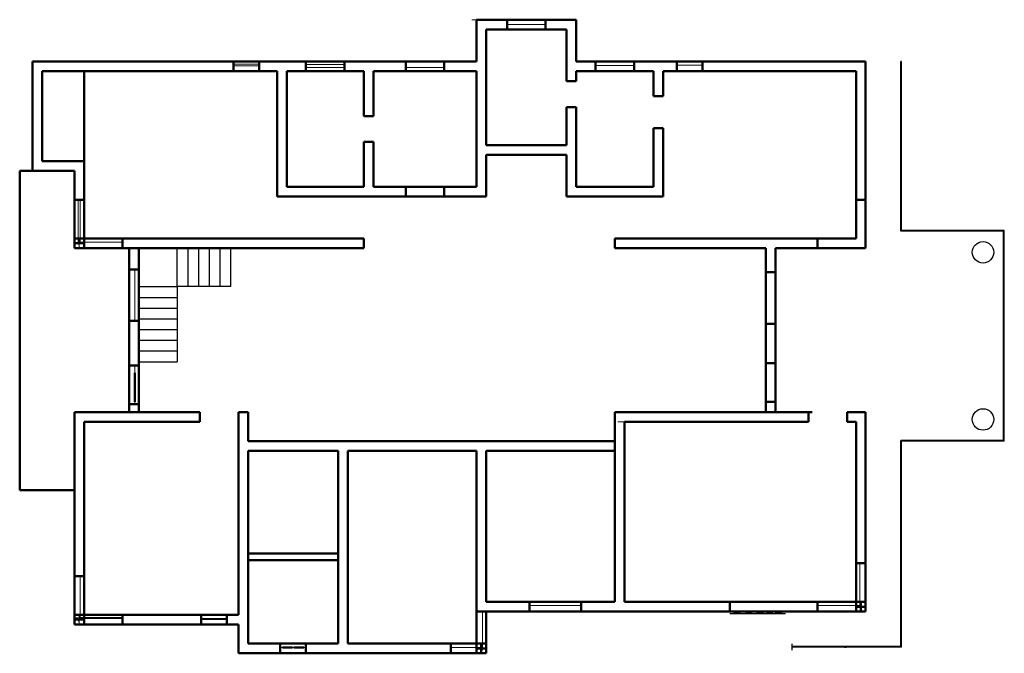
# Model space of a CAD drawing. Units: inches. Extents: x -3 to 916, y -523 to 68.
import ezdxf

# ---------------------------------------------------------------- set-up
doc = ezdxf.new("R2010")
doc.units = ezdxf.units.IN
doc.header["$MEASUREMENT"] = 0
for name, color, linetype, lineweight in [('A-DOOR', 3, 'Continuous', 25), ('A-FLOR-STRS', 2, 'Continuous', 25), ('A-GLAZ', 4, 'Continuous', 18), ('A-WALL', 7, 'Continuous', 50), ('C-PROP', 8, 'Continuous', 25)]:
    doc.layers.add(name, color=color, linetype=linetype, lineweight=lineweight)

msp = doc.modelspace()

# ---------------------------------------------------------------- linework, layer by layer
at = {"layer": 'A-DOOR', "extrusion": (0, -1, 0)}
for p, q in [((663.4, -485.93, 91.57), (669.77, -485.93, 91.57)), ((669.77, -485.93, 33.07), (663.4, -485.93, 33.07)), ((663.4, -485.93, 33.07), (663.4, -485.93, 91.57)), ((669.77, -485.93, 91.57), (669.77, -485.93, 33.07)), ((674.29, -485.93, 91.57), (680.65, -485.93, 91.57)), ((680.65, -485.93, 33.07), (674.29, -485.93, 33.07)), ((674.29, -485.93, 33.07), (674.29, -485.93, 91.57)), ((680.65, -485.93, 91.57), (680.65, -485.93, 33.07)), ((684.71, -485.93, 91.57), (691.07, -485.93, 91.57)), ((691.07, -485.93, 33.07), (684.71, -485.93, 33.07)), ((684.71, -485.93, 33.07), (684.71, -485.93, 91.57)), ((691.07, -485.93, 91.57), (691.07, -485.93, 33.07)), ((699.91, -485.93, 91.57), (693.92, -485.93, 91.57)), ((693.92, -485.93, 91.57), (693.92, -485.93, 33.07)), ((693.92, -485.93, 33.07), (699.91, -485.93, 33.07)), ((699.91, -485.93, 33.07), (699.91, -485.93, 91.57)), ((702.1, -485.93, 91.57), (708.47, -485.93, 91.57)), ((708.47, -485.93, 33.07), (702.1, -485.93, 33.07)), ((702.1, -485.93, 33.07), (702.1, -485.93, 91.57)), ((708.47, -485.93, 91.57), (708.47, -485.93, 33.07))]:
    msp.add_line(p, q, dxfattribs=at)
at = {"layer": 'A-DOOR', "extrusion": (6.6e-15, 1, 1.128e-12)}
msp.add_open_spline([(659.86, -485.93, 180), (668.48, -485.93, 174.09), (685.72, -485.93, 162.26), (702.96, -485.93, 174.09), (711.58, -485.93, 180)], degree=3, dxfattribs=at)
at = {"layer": 'A-FLOR-STRS'}
for p, q in [((144.44, -180.93), (144.44, -144.93)), ((154.44, -180.93), (154.44, -144.93)), ((164.44, -180.93), (164.44, -144.93)), ((174.44, -180.93), (174.44, -144.93)), ((184.44, -180.93), (184.44, -144.93)), ((194.44, -180.93), (194.44, -144.93)), ((108.44, -180.93), (144.44, -180.93)), ((194.44, -180.93), (144.44, -180.93)), ((144.44, -180.93), (144.44, -250.93)), ((108.44, -190.93), (144.44, -190.93)), ((108.44, -200.93), (144.44, -200.93)), ((108.44, -210.93), (144.44, -210.93)), ((108.44, -220.93), (144.44, -220.93)), ((108.44, -230.93), (144.44, -230.93)), ((108.44, -240.93), (144.44, -240.93)), ((108.44, -250.93), (144.44, -250.93))]:
    msp.add_line(p, q, dxfattribs=at)
at = {"layer": 'A-GLAZ'}
for p, q in [((52.94, -135.93, 150), (52.94, -144.93, 150)), ((51.94, -140.43, 150), (51.94, -141.43, 150)), ((51.94, -141.43, 150), (52.94, -141.43, 150)), ((781.94, -480.43, 36), (782.94, -480.43, 36)), ((782.94, -480.43, 36), (782.94, -479.43, 36)), ((52.94, -486.93, 36), (52.94, -495.93, 36)), ((52.94, -486.93, 150), (52.94, -495.93, 150))]:
    msp.add_line(p, q, dxfattribs=at)
at = {"layer": 'A-GLAZ', "extrusion": (1, 0, 0)}
msp.add_line((52.94, -135.93, 36), (52.94, -144.93, 36), dxfattribs=at)
at = {"layer": 'A-GLAZ', "extrusion": (-3e-16, -1, 0)}
for points, elevation in [([(419.07, 60), (427.82, 60), (427.82, 38.81), (419.07, 38.81)], -68.07), ([(423.44, 60), (432.2, 60), (432.2, 38.81), (423.44, 38.81)], -68.07), ([(555.44, 52.29), (564.19, 52.29), (564.19, 31.1), (555.44, 31.1)], 306.93), ([(557.07, 52.29), (565.82, 52.29), (565.82, 31.1), (557.07, 31.1)], 306.93), ([(455.82, 146.15), (464.57, 146.15), (464.57, 124.96), (455.82, 124.96)], 483.93), ([(468.97, 146.15), (477.73, 146.15), (477.73, 124.96), (468.97, 124.96)], 483.93), ([(481.71, 146.15), (490.46, 146.15), (490.46, 124.96), (481.71, 124.96)], 483.93), ([(493.74, 146.15), (502.5, 146.15), (502.5, 124.96), (493.74, 124.96)], 483.93), ([(506.54, 146.15), (515.29, 146.15), (515.29, 124.96), (506.54, 124.96)], 483.93), ([(519.12, 146.15), (527.87, 146.15), (527.87, 124.96), (519.12, 124.96)], 483.93), ([(531.8, 146.15), (540.56, 146.15), (540.56, 124.96), (531.8, 124.96)], 483.93), ([(544.87, 146.15), (553.62, 146.15), (553.62, 124.96), (544.87, 124.96)], 483.93), ([(557.89, 146.15), (566.64, 146.15), (566.64, 124.96), (557.89, 124.96)], 483.93)]:
    msp.add_lwpolyline(points, close=True, dxfattribs=dict(at, elevation=elevation))
at = {"layer": 'A-GLAZ', "extrusion": (0, 1, 0)}
for points, elevation in [([(-487.94, 90), (-487.94, 36), (-451.94, 36), (-451.94, 90)], 63.7), ([(-485.94, 88), (-485.94, 38), (-453.94, 38), (-453.94, 88)], 63.7), ([(-220.82, 90), (-220.82, 36), (-196.82, 36), (-196.82, 90)], 26.44), ([(-218.82, 88), (-218.82, 38), (-198.82, 38), (-198.82, 88)], 26.44), ([(-300.44, 210), (-300.44, 150), (-264.44, 150), (-264.44, 210)], 26.39), ([(-300.44, 90), (-300.44, 36), (-264.44, 36), (-264.44, 90)], 23.57), ([(-298.44, 208), (-298.44, 152), (-266.44, 152), (-266.44, 208)], 26.39), ([(-298.44, 88), (-298.44, 38), (-266.44, 38), (-266.44, 88)], 23.57), ([(-393.44, 90), (-393.44, 36), (-357.44, 36), (-357.44, 90)], 23.57), ([(-391.44, 88), (-391.44, 38), (-359.44, 38), (-359.44, 88)], 23.57), ([(-570.44, 90), (-570.44, 36), (-534.44, 36), (-534.44, 90)], 25.47), ([(-568.44, 88), (-568.44, 38), (-536.44, 38), (-536.44, 88)], 25.47), ([(-634.22, 90), (-634.22, 36), (-610.22, 36), (-610.22, 90)], 25.52), ([(-632.22, 88), (-632.22, 38), (-612.22, 38), (-612.22, 88)], 25.52), ([(-54.94, 208), (-73.19, 208), (-73.19, 152), (-54.94, 152)], -139.43), ([(-55.94, 207), (-72.19, 207), (-72.19, 153), (-55.94, 153)], -139.43), ([(-73.19, 208), (-91.44, 208), (-91.44, 152), (-73.19, 152)], -139.43), ([(-474.98, 88), (-496.98, 88), (-496.98, 38), (-474.98, 38)], -478.43), ([(-475.98, 87), (-495.98, 87), (-495.98, 39), (-475.98, 39)], -478.43), ([(-497.06, 88), (-519.06, 88), (-519.06, 38), (-497.06, 38)], -478.43), ([(-498.06, 87), (-518.06, 87), (-518.06, 39), (-498.06, 39)], -478.43)]:
    msp.add_lwpolyline(points, close=True, dxfattribs=dict(at, elevation=elevation))
at = {"layer": 'A-GLAZ', "extrusion": (0, -1, 0)}
for points, elevation in [([(469.94, 88), (453.94, 88), (453.94, 38), (469.94, 38)], -63.7), ([(468.94, 87), (454.94, 87), (454.94, 39), (468.94, 39)], -63.7), ([(485.94, 88), (469.94, 88), (469.94, 38), (485.94, 38)], -63.7), ([(484.94, 87), (470.94, 87), (470.94, 39), (484.94, 39)], -63.7), ([(208.82, 88), (198.82, 88), (198.82, 38), (208.82, 38)], -26.44), ([(207.82, 87), (199.82, 87), (199.82, 39), (207.82, 39)], -26.44), ([(218.82, 88), (208.82, 88), (208.82, 38), (218.82, 38)], -26.44), ([(217.82, 87), (209.82, 87), (209.82, 39), (217.82, 39)], -26.44), ([(282.44, 208), (266.44, 208), (266.44, 152), (282.44, 152)], -26.39), ([(282.44, 88), (266.44, 88), (266.44, 38), (282.44, 38)], -23.57), ([(281.44, 207), (267.44, 207), (267.44, 153), (281.44, 153)], -26.39), ([(281.44, 87), (267.44, 87), (267.44, 39), (281.44, 39)], -23.57), ([(298.44, 208), (282.44, 208), (282.44, 152), (298.44, 152)], -26.39), ([(298.44, 88), (282.44, 88), (282.44, 38), (298.44, 38)], -23.57), ([(297.44, 207), (283.44, 207), (283.44, 153), (297.44, 153)], -26.39), ([(297.44, 87), (283.44, 87), (283.44, 39), (297.44, 39)], -23.57), ([(375.44, 88), (359.44, 88), (359.44, 38), (375.44, 38)], -23.57), ([(374.44, 87), (360.44, 87), (360.44, 39), (374.44, 39)], -23.57), ([(391.44, 88), (375.44, 88), (375.44, 38), (391.44, 38)], -23.57), ([(390.44, 87), (376.44, 87), (376.44, 39), (390.44, 39)], -23.57), ([(552.44, 88), (536.44, 88), (536.44, 38), (552.44, 38)], -25.47), ([(551.44, 87), (537.44, 87), (537.44, 39), (551.44, 39)], -25.47), ([(568.44, 88), (552.44, 88), (552.44, 38), (568.44, 38)], -25.47), ([(567.44, 87), (553.44, 87), (553.44, 39), (567.44, 39)], -25.47), ([(622.22, 88), (612.22, 88), (612.22, 38), (622.22, 38)], -25.52), ([(621.22, 87), (613.22, 87), (613.22, 39), (621.22, 39)], -25.52), ([(632.22, 88), (622.22, 88), (622.22, 38), (632.22, 38)], -25.52), ([(631.22, 87), (623.22, 87), (623.22, 39), (631.22, 39)], -25.52), ([(93.44, 210), (93.44, 150), (52.94, 150), (52.94, 210)], 139.43), ([(91.44, 208), (91.44, 152), (54.94, 152), (54.94, 208)], 139.43), ([(472.98, 90), (472.98, 36), (520.98, 36), (520.98, 90)], 478.43), ([(474.98, 88), (474.98, 38), (518.98, 38), (518.98, 88)], 478.43), ([(741.44, 90), (781.94, 90), (781.94, 36), (741.44, 36)], 478.43), ([(743.44, 88), (779.94, 88), (779.94, 38), (743.44, 38)], 478.43), ([(743.44, 88), (761.69, 88), (761.69, 38), (743.44, 38)], 478.43), ([(744.44, 87), (760.69, 87), (760.69, 39), (744.44, 39)], 478.43), ([(761.69, 88), (779.94, 88), (779.94, 38), (761.69, 38)], 478.43), ([(762.69, 87), (778.94, 87), (778.94, 39), (762.69, 39)], 478.43), ([(52.94, 90), (93.44, 90), (93.44, 36), (52.94, 36)], 489.56), ([(54.94, 88), (91.44, 88), (91.44, 38), (54.94, 38)], 489.56), ([(54.94, 88), (73.19, 88), (73.19, 38), (54.94, 38)], 489.56), ([(55.94, 87), (72.19, 87), (72.19, 39), (55.94, 39)], 489.56), ([(73.19, 88), (91.44, 88), (91.44, 38), (73.19, 38)], 489.56), ([(74.19, 87), (90.44, 87), (90.44, 39), (74.19, 39)], 489.56), ([(190.66, 210), (190.66, 150), (166.66, 150), (166.66, 210)], 490.43), ([(166.66, 90), (166.66, 36), (190.66, 36), (190.66, 90)], 491.43), ([(188.66, 208), (188.66, 152), (168.66, 152), (168.66, 208)], 490.43), ([(168.66, 88), (168.66, 38), (188.66, 38), (188.66, 88)], 491.43), ([(187.66, 207), (187.66, 153), (169.66, 153), (169.66, 207)], 490.43), ([(169.66, 87), (169.66, 39), (187.66, 39), (187.66, 87)], 491.43), ([(240.44, 114), (240.44, 96), (264.44, 96), (264.44, 114)], 517.43), ([(242.44, 112), (242.44, 98), (262.44, 98), (262.44, 112)], 517.43), ([(399.44, 90), (399.44, 36), (427.94, 36), (427.94, 90)], 517.43), ([(401.44, 88), (401.44, 38), (425.94, 38), (425.94, 88)], 517.43)]:
    msp.add_lwpolyline(points, close=True, dxfattribs=dict(at, elevation=elevation))
at = {"layer": 'A-GLAZ', "extrusion": (7e-16, 1, 0), "elevation": 24.96}
for points in [[(-220.82, 210), (-220.82, 150), (-196.82, 150), (-196.82, 210)], [(-218.82, 208), (-218.82, 152), (-198.82, 152), (-198.82, 208)], [(-217.82, 207), (-217.82, 153), (-199.82, 153), (-199.82, 207)]]:
    msp.add_lwpolyline(points, close=True, dxfattribs=at)
at = {"layer": 'A-GLAZ', "extrusion": (-1, 0, 0)}
for points, elevation in [([(99.93, 210), (99.93, 150), (140.43, 150), (140.43, 210)], -51.94), ([(99.93, 90), (140.43, 90), (140.43, 36), (99.93, 36)], -53.94), ([(101.93, 208), (101.93, 152), (138.43, 152), (138.43, 208)], -51.94), ([(101.93, 88), (138.43, 88), (138.43, 38), (101.93, 38)], -53.94), ([(164.82, 210), (164.82, 150), (212.82, 150), (212.82, 210)], -104.94), ([(166.82, 208), (166.82, 152), (210.82, 152), (210.82, 208)], -104.94), ([(254.43, 150), (254.43, 210), (290.43, 210), (290.43, 150)], -104.94), ([(256.43, 152), (256.43, 208), (288.43, 208), (288.43, 152)], -104.94), ([(450.93, 210), (450.93, 150), (491.43, 150), (491.43, 210)], -53.94), ([(452.93, 208), (452.93, 152), (489.43, 152), (489.43, 208)], -53.94), ([(453.93, 207), (453.93, 153), (488.43, 153), (488.43, 207)], -53.94)]:
    msp.add_lwpolyline(points, close=True, dxfattribs=dict(at, elevation=elevation))
at = {"layer": 'A-GLAZ', "extrusion": (1, 0, 0)}
for points, elevation in [([(-101.93, 208), (-120.18, 208), (-120.18, 152), (-101.93, 152)], 51.94), ([(-102.93, 207), (-119.18, 207), (-119.18, 153), (-102.93, 153)], 51.94), ([(-101.93, 88), (-120.18, 88), (-120.18, 38), (-101.93, 38)], 53.94), ([(-102.93, 87), (-119.18, 87), (-119.18, 39), (-102.93, 39)], 53.94), ([(-120.18, 88), (-138.43, 88), (-138.43, 38), (-120.18, 38)], 53.94), ([(-121.18, 87), (-137.43, 87), (-137.43, 39), (-121.18, 39)], 53.94), ([(-166.82, 208), (-188.82, 208), (-188.82, 152), (-166.82, 152)], 104.94), ([(-167.82, 207), (-187.82, 207), (-187.82, 153), (-167.82, 153)], 104.94), ([(-188.82, 208), (-210.82, 208), (-210.82, 152), (-188.82, 152)], 104.94), ([(-189.82, 207), (-209.82, 207), (-209.82, 153), (-189.82, 153)], 104.94), ([(-256.43, 208), (-272.43, 208), (-272.43, 152), (-256.43, 152)], 104.94), ([(-257.43, 207), (-271.43, 207), (-271.43, 153), (-257.43, 153)], 104.94), ([(-272.43, 208), (-288.43, 208), (-288.43, 152), (-272.43, 152)], 104.94), ([(-273.43, 207), (-287.43, 207), (-287.43, 153), (-273.43, 153)], 104.94), ([(-438.93, 90), (-438.93, 36), (-479.43, 36), (-479.43, 90)], 780.94), ([(-518.43, 36), (-483.93, 36), (-483.93, 90), (-518.43, 90)], 428.94), ([(-516.43, 38), (-485.93, 38), (-485.93, 88), (-516.43, 88)], 428.94)]:
    msp.add_lwpolyline(points, close=True, dxfattribs=dict(at, elevation=elevation))
at = {"layer": 'A-GLAZ', "extrusion": (-1, 3e-16, 0), "elevation": -104.94}
for points in [[(254.43, 90), (254.43, 0), (290.43, 0), (290.43, 90)], [(256.43, 88), (256.43, 2), (288.43, 2), (288.43, 88)]]:
    msp.add_lwpolyline(points, close=True, dxfattribs=at)
at = {"layer": 'A-GLAZ', "extrusion": (1, 0, 0), "elevation": 780.94}
for points in [[(-456.78, 88), (-440.93, 88), (-440.93, 38), (-456.78, 38)], [(-455.58, 87), (-441.93, 87), (-441.93, 39), (-455.58, 39)], [(-456.78, 38), (-477.43, 38), (-477.43, 88), (-456.78, 88)], [(-456.78, 39), (-476.43, 39), (-476.43, 87), (-456.78, 87)]]:
    msp.add_lwpolyline(points, dxfattribs=at)
at = {"layer": 'A-GLAZ', "extrusion": (-1, 3.2e-15, 0), "elevation": -53.94}
for points in [[(450.93, 90), (450.93, 36), (490.56, 36), (490.56, 90)], [(452.93, 88), (452.93, 38), (488.56, 38), (488.56, 88)], [(453.93, 87), (453.93, 39), (487.56, 39), (487.56, 87)]]:
    msp.add_lwpolyline(points, close=True, dxfattribs=at)
at = {"layer": 'A-GLAZ', "extrusion": (-1, -6.3e-15, 0), "elevation": -428.94}
for points in [[(501.18, 88), (485.93, 88), (485.93, 38), (501.18, 38)], [(500.18, 87), (486.93, 87), (486.93, 39), (500.18, 39)], [(516.43, 88), (501.18, 88), (501.18, 38), (516.43, 38)], [(515.43, 87), (502.18, 87), (502.18, 39), (515.43, 39)]]:
    msp.add_lwpolyline(points, close=True, dxfattribs=at)
at = {"layer": 'A-GLAZ', "extrusion": (8e-16, -1, 0), "elevation": 490.43}
for points in [[(93.44, 210), (93.44, 150), (52.94, 150), (52.94, 210)], [(91.44, 208), (91.44, 152), (54.94, 152), (54.94, 208)]]:
    msp.add_lwpolyline(points, close=True, dxfattribs=at)
for points in [[(76.67, 153), (55.94, 153), (55.94, 207), (76.67, 207)], [(77.67, 207), (90.44, 207), (90.44, 153), (77.67, 153)]]:
    msp.add_lwpolyline(points, dxfattribs=at)
at = {"layer": 'A-GLAZ', "extrusion": (-6.4e-15, 1, 0), "elevation": -517.43}
for points in [[(-401.44, 88), (-413.69, 88), (-413.69, 38), (-401.44, 38)], [(-402.44, 87), (-412.69, 87), (-412.69, 39), (-402.44, 39)]]:
    msp.add_lwpolyline(points, close=True, dxfattribs=at)
at = {"layer": 'A-WALL'}
for p, q in [((423.44, 68.07), (423.44, 29.07)), ((423.44, 68.07), (516.44, 68.07)), ((451.94, 59.07), (451.94, 68.07)), ((487.94, 59.07), (487.94, 68.07)), ((516.44, 68.07), (516.44, 29.07)), ((432.44, 59.07), (432.44, -48.93)), ((432.44, 59.07), (507.44, 59.07)), ((507.44, 59.07), (507.44, 10.62)), ((9.44, 29.07), (423.44, 29.07)), ((9.44, 29.07), (9.44, -72.93)), ((196.82, 29.07), (196.82, 20.07)), ((220.82, 29.07), (220.82, 20.07)), ((264.44, 20.07), (264.44, 29.07)), ((300.44, 20.07), (300.44, 29.07)), ((357.44, 20.07), (357.44, 29.07)), ((393.44, 20.07), (393.44, 29.07)), ((516.44, 29.07), (786.44, 29.07)), ((534.44, 20.07), (534.44, 29.07)), ((570.44, 20.07), (570.44, 29.07)), ((610.22, 29.07), (610.22, 20.07)), ((634.22, 29.07), (634.22, 20.07)), ((786.44, 29.07), (786.44, -144.93)), ((18.44, 20.07), (57.44, 20.07)), ((18.44, 20.07), (18.44, -63.93)), ((57.44, 20.07), (57.44, -135.93)), ((57.44, 20.07), (237.44, 20.07)), ((237.44, 20.07), (237.44, -96.93)), ((246.44, 20.07), (246.44, -87.93)), ((246.44, 20.07), (318.44, 20.07)), ((318.44, 20.07), (318.44, -21.93)), ((327.44, 20.07), (327.44, -21.93)), ((327.44, 20.07), (423.44, 20.07)), ((423.44, 20.07), (423.44, -87.93)), ((516.44, 20.07), (588.44, 20.07)), ((516.44, 20.07), (516.44, 10.62)), ((588.44, 20.07), (588.44, -3.26)), ((597.44, 20.07), (597.44, -3.26)), ((597.44, 20.07), (777.44, 20.07)), ((777.44, 20.07), (777.44, -135.93)), ((516.44, 10.62), (507.44, 10.62)), ((588.44, -3.26), (597.44, -3.26)), ((516.44, -13.38), (507.44, -13.38)), ((507.44, -13.38), (507.44, -48.93)), ((516.44, -13.38), (516.44, -87.93)), ((327.44, -21.93), (318.44, -21.93)), ((588.44, -33.26), (597.44, -33.26)), ((588.44, -33.26), (588.44, -87.93)), ((597.44, -33.26), (597.44, -96.93)), ((327.44, -45.93), (318.44, -45.93)), ((318.44, -45.93), (318.44, -87.93)), ((327.44, -45.93), (327.44, -87.93)), ((432.44, -48.93), (507.44, -48.93)), ((18.44, -63.93), (57.44, -63.93)), ((432.44, -57.93), (507.44, -57.93)), ((432.44, -57.93), (432.44, -96.93)), ((507.44, -57.93), (507.44, -96.93)), ((9.44, -72.93), (-2.56, -72.93)), ((-2.56, -72.93), (-2.56, -370.7)), ((9.44, -72.93), (48.44, -72.93)), ((48.44, -72.93), (48.44, -144.93)), ((246.44, -87.93), (318.44, -87.93)), ((327.44, -87.93), (423.44, -87.93)), ((357.44, -87.93), (357.44, -96.93)), ((393.44, -87.93), (393.44, -96.93)), ((516.44, -87.93), (588.44, -87.93)), ((57.44, -99.93), (48.44, -99.93)), ((237.44, -96.93), (432.44, -96.93)), ((507.44, -96.93), (597.44, -96.93)), ((777.44, -99.93), (786.44, -99.93)), ((57.44, -135.93, 150), (48.44, -135.93, 150)), ((57.44, -135.93), (318.44, -135.93)), ((57.44, -135.93), (237.44, -135.93)), ((57.44, -135.93, 150), (57.44, -144.93, 150)), ((57.44, -135.93, 36), (57.44, -144.93, 36)), ((93.44, -135.93), (93.44, -144.93)), ((318.44, -135.93), (318.44, -144.93)), ((552.44, -144.93), (552.44, -135.93)), ((552.44, -135.93), (777.44, -135.93)), ((741.44, -135.93), (741.44, -144.93)), ((57.44, -140.43, 150), (48.44, -140.43, 150)), ((48.44, -144.93), (150.44, -144.93)), ((99.44, -144.93), (99.44, -297.93)), ((108.44, -144.93), (108.44, -297.93)), ((150.44, -144.93), (318.44, -144.93)), ((552.44, -144.93), (693.44, -144.93)), ((693.44, -144.93), (693.44, -252.27)), ((702.44, -144.93), (702.44, -252.27)), ((702.44, -144.93), (786.44, -144.93)), ((108.44, -164.82), (99.44, -164.82)), ((693.44, -167.49), (702.44, -167.49)), ((108.44, -212.82), (99.44, -212.82)), ((693.44, -215.49), (702.44, -215.49)), ((99.44, -254.43), (108.44, -254.43)), ((702.44, -252.27), (693.44, -252.27)), ((99.44, -290.43), (108.44, -290.43)), ((702.44, -288.27), (693.44, -288.27)), ((693.44, -288.27), (693.44, -297.93)), ((702.44, -288.27), (702.44, -297.93)), ((48.44, -297.93), (48.44, -495.93)), ((48.44, -297.93), (99.44, -297.93)), ((99.44, -297.93), (108.44, -297.93)), ((108.44, -297.93), (150.44, -297.93)), ((150.44, -297.93), (165.44, -297.93)), ((165.44, -306.93), (165.44, -297.93)), ((201.44, -306.93), (201.44, -297.93)), ((201.44, -297.93), (210.44, -297.93)), ((210.44, -297.93), (210.44, -324.93)), ((552.44, -297.93), (552.44, -474.93)), ((552.44, -297.93), (693.44, -297.93)), ((702.44, -297.93), (693.44, -297.93)), ((702.44, -297.93), (733.21, -297.93)), ((733.21, -306.93), (733.21, -297.93)), ((769.21, -306.93), (769.21, -297.93)), ((769.21, -297.93), (786.44, -297.93)), ((786.44, -297.93, 14.59), (786.44, -483.93, 14.59)), ((786.44, -297.93, 14.59), (786.44, -297.93, 12.59)), ((786.44, -297.93, 12.59), (786.44, -483.93, 12.59)), ((57.44, -306.93), (57.44, -486.93)), ((57.44, -306.93), (165.44, -306.93)), ((201.44, -306.93), (201.44, -486.93)), ((561.44, -306.93), (561.44, -474.93)), ((561.44, -306.93), (733.21, -306.93)), ((769.21, -306.93), (777.44, -306.93)), ((777.44, -306.93), (777.44, -474.93)), ((210.44, -324.93), (552.44, -324.93)), ((210.44, -333.93), (294.44, -333.93)), ((210.44, -333.93), (210.44, -513.93)), ((294.44, -333.93), (294.44, -513.93)), ((303.44, -333.93), (303.44, -513.93)), ((303.44, -333.93), (423.44, -333.93)), ((423.44, -333.93), (423.44, -513.93)), ((432.44, -333.93), (432.44, -474.93)), ((432.44, -333.93), (552.44, -333.93)), ((786.44, -333.93), (786.44, -483.93)), ((-2.56, -370.7), (48.44, -370.7)), ((210.44, -429.93), (294.44, -429.93)), ((210.44, -435.93), (294.44, -435.93)), ((777.44, -438.93), (786.44, -438.93)), ((57.44, -450.93), (48.44, -450.93)), ((432.44, -474.93), (552.44, -474.93)), ((472.98, -474.93), (472.98, -483.93)), ((520.98, -474.93), (520.98, -483.93)), ((561.44, -474.93), (777.44, -474.93)), ((741.44, -474.93), (741.44, -483.93)), ((777.44, -474.93, 36), (777.44, -483.93, 36)), ((781.94, -474.93, 36), (781.94, -483.93, 36)), ((432.44, -483.93), (423.44, -483.93)), ((432.44, -483.93), (786.44, -483.93)), ((432.44, -483.93), (432.44, -522.93)), ((777.44, -479.43, 36), (786.44, -479.43, 36)), ((57.44, -486.93, 150), (48.44, -486.93, 150)), ((57.44, -490.56, 36), (48.44, -490.56, 36)), ((57.44, -491.43, 150), (48.44, -491.43, 150)), ((51.94, -491.56, 36), (51.94, -490.56, 36)), ((51.94, -491.43, 150), (51.94, -492.43, 150)), ((52.94, -491.56, 36), (51.94, -491.56, 36)), ((51.94, -492.43, 150), (52.94, -492.43, 150)), ((57.44, -486.93), (201.44, -486.93)), ((57.44, -486.93, 36), (57.44, -495.93, 36)), ((57.44, -486.93, 150), (57.44, -495.93, 150)), ((93.44, -486.93), (93.44, -495.93)), ((166.66, -486.93), (166.66, -495.93)), ((190.66, -486.93), (190.66, -495.93)), ((48.44, -495.93), (201.44, -495.93)), ((201.44, -495.93), (201.44, -522.93)), ((210.44, -513.93), (294.44, -513.93)), ((210.44, -513.93), (294.44, -513.93)), ((240.44, -513.93), (240.44, -522.93)), ((264.44, -513.93), (264.44, -522.93)), ((303.44, -513.93), (423.44, -513.93)), ((399.44, -513.93), (399.44, -522.93)), ((423.44, -513.93, 36), (423.44, -522.93, 36)), ((427.94, -513.93, 36), (427.94, -522.93, 36)), ((201.44, -522.93), (432.44, -522.93)), ((423.44, -518.43, 36), (432.44, -518.43, 36)), ((427.94, -519.43, 36), (428.94, -519.43, 36)), ((428.94, -519.43, 36), (428.94, -518.43, 36))]:
    msp.add_line(p, q, dxfattribs=at)
at = {"layer": 'A-WALL', "extrusion": (1, 0, 0)}
for p, q in [((57.44, -135.93, 36), (48.44, -135.93, 36)), ((57.44, -140.43, 36), (48.44, -140.43, 36)), ((57.44, -144.93, 36), (57.44, -140.43, 36)), ((104.94, -288.43, 88), (104.94, -261.35, 85.62)), ((104.94, -261.35, 85.62), (104.94, -261.35, 7.65)), ((104.94, -261.35, 7.65), (104.94, -288.43, 2)), ((786.44, -297.93, 25.13), (786.44, -483.93, 25.13)), ((786.44, -297.93, 33.36), (786.44, -483.93, 33.36)), ((786.44, -483.93, 35.36), (786.44, -297.93, 35.36)), ((786.44, -297.93, 43.9), (786.44, -438.93, 43.9)), ((786.44, -438.93, 45.9), (786.44, -297.93, 45.9)), ((786.44, -297.93, 69.62), (786.44, -438.93, 69.62)), ((786.44, -438.93, 71.62), (786.44, -297.93, 71.62)), ((786.44, -438.93, 43.9), (786.44, -438.93, 45.9)), ((786.44, -438.93, 69.62), (786.44, -438.93, 71.62)), ((659.86, -483.93, 156), (659.86, -474.93, 156)), ((711.58, -483.93), (659.86, -483.93)), ((659.86, -483.93), (659.86, -483.93, 156)), ((741.41, -483.93, 35.36), (711.58, -483.93, 35.36)), ((741.44, -483.93, 67.3), (711.58, -483.93, 67.3)), ((711.58, -483.93, 67.3), (711.58, -483.93, 69.3)), ((711.58, -483.93, 69.3), (741.44, -483.93, 69.3)), ((786.44, -483.93, 33.36), (741.41, -483.93, 33.36)), ((741.41, -483.93, 33.36), (741.41, -483.93, 35.36)), ((741.41, -483.93, 35.36), (786.44, -483.93, 35.36))]:
    msp.add_line(p, q, dxfattribs=at)
at = {"layer": 'A-WALL', "extrusion": (0, 1, 0)}
for p, q in [((693.44, -288.27), (693.44, -252.27)), ((57.44, -486.93, 36), (48.44, -486.93, 36)), ((76.67, -490.43, 207), (76.67, -490.43, 153)), ((77.67, -490.43, 207), (77.67, -490.43, 153)), ((251.84, -517.43, 104.4), (242.44, -517.43, 104.4)), ((251.84, -517.43, 105.6), (242.44, -517.43, 105.6)), ((251.84, -517.43, 112), (251.84, -517.43, 105.6)), ((251.84, -517.43, 104.4), (251.84, -517.43, 98)), ((262.44, -517.43, 105.6), (253.04, -517.43, 105.6)), ((262.44, -517.43, 104.4), (253.04, -517.43, 104.4)), ((253.04, -517.43, 112), (253.04, -517.43, 105.6)), ((253.04, -517.43, 104.4), (253.04, -517.43, 98))]:
    msp.add_line(p, q, dxfattribs=at)
at = {"layer": 'A-WALL', "extrusion": (0, -1, 0)}
for p, q in [((702.44, -252.27), (702.44, -288.27)), ((730.03, -297.93, 16.77), (736.4, -297.93, 16.77)), ((730.03, -297.93, 16.77), (736.4, -297.93, 16.77)), ((730.03, -297.93, 16.77), (736.4, -297.93, 16.77)), ((730.03, -297.93, 16.77), (736.4, -297.93, 16.77)), ((786.44, -483.93, 23.13), (786.44, -297.96, 23.13)), ((777.44, -474.93, 36), (786.44, -474.93, 36)), ((741.44, -483.93, 25.13), (711.58, -483.93, 25.13)), ((741.44, -483.93, 23.13), (711.58, -483.93, 23.13)), ((741.44, -483.93, 33.36), (711.58, -483.93, 33.36)), ((786.44, -483.93, 25.13), (741.44, -483.93, 25.13)), ((741.44, -483.93, 25.13), (741.44, -483.93, 23.13)), ((741.44, -483.93, 23.13), (786.44, -483.93, 23.13)), ((423.44, -513.93, 36), (432.44, -513.93, 36))]:
    msp.add_line(p, q, dxfattribs=at)
at = {"layer": 'A-WALL', "extrusion": (1, 5e-15, 0)}
for p, q in [((786.44, -297.93, 56.18), (786.44, -438.93, 56.18)), ((786.44, -438.93, 58.18), (786.44, -297.93, 58.18)), ((786.44, -297.93, 80.91), (786.44, -438.93, 80.91)), ((786.44, -438.93, 82.91), (786.44, -297.93, 82.91)), ((786.44, -297.93, 91.46), (786.44, -438.93, 91.46)), ((786.44, -437.93, 92.46), (786.44, -297.93, 92.46)), ((786.44, -438.93, 91.46), (786.44, -437.93, 91.46)), ((786.44, -437.93, 91.46), (786.44, -437.93, 92.46)), ((786.44, -438.93, 56.18), (786.44, -438.93, 58.18)), ((786.44, -438.93, 80.91), (786.44, -438.93, 82.91))]:
    msp.add_line(p, q, dxfattribs=at)
at = {"layer": 'A-WALL', "extrusion": (-1, -2.7e-15, 0)}
for p, q in [((780.94, -455.58, 87), (780.94, -455.58, 39)), ((780.94, -455.58, 87), (780.94, -455.58, 39)), ((780.94, -456.78, 87), (780.94, -456.78, 39))]:
    msp.add_line(p, q, dxfattribs=at)
at = {"layer": 'A-WALL', "extrusion": (1, 1.26e-14, 0)}
for p, q in [((741.44, -483.93, 79.23), (711.49, -483.93, 79.23)), ((711.49, -483.93, 81.23), (741.44, -483.93, 81.23)), ((741.44, -483.93, 43.95), (711.58, -483.93, 43.95)), ((711.58, -483.93, 43.95), (711.58, -483.93, 45.95)), ((711.58, -483.93, 45.95), (741.44, -483.93, 45.95)), ((711.58, -483.93, 79.23), (711.58, -483.93, 81.23)), ((741.44, -483.93, 56.25), (711.61, -483.93, 56.25)), ((711.61, -483.93, 56.25), (711.61, -483.93, 58.25)), ((711.61, -483.93, 58.25), (741.44, -483.93, 58.25))]:
    msp.add_line(p, q, dxfattribs=at)
at = {"layer": 'A-WALL', "extrusion": (-1, 0, 0)}
msp.add_line((711.58, -483.93, 114), (711.58, -483.93), dxfattribs=at)
at = {"layer": 'A-WALL', "extrusion": (6.3e-15, -1, 0), "elevation": 483.93}
msp.add_lwpolyline([(432.44, 90), (432.44, 36), (432.44, 36), (432.44, 90)], close=True, dxfattribs=at)
msp.add_lwpolyline([(432.44, 90), (432.44, 36), (432.44, 36), (432.44, 90)], close=True, dxfattribs=at)
at = {"layer": 'A-WALL', "extrusion": (-1, 0, 0), "elevation": -93.44}
msp.add_lwpolyline([(495.93, 210), (495.93, 150), (495.93, 150), (495.93, 210)], close=True, dxfattribs=at)
at = {"layer": 'C-PROP', "extrusion": (0, 0, -1)}
for p, q in [((819.14, -129.11, 132), (819.14, 29.06, 132)), ((819.74, 28.79, 132), (819.14, 28.79, 132)), ((819.74, -128.51, 132), (819.74, 29.06, 132)), ((819.14, 8.55, 132), (819.74, 8.55, 132)), ((819.74, -2.15, 132), (819.14, -2.15, 132)), ((819.74, -22.94, 132), (819.14, -22.94, 132)), ((819.74, -43.14, 132), (819.14, -43.14, 132)), ((819.74, -128.51, 132), (819.14, -128.51, 132)), ((915.74, -128.51, 132), (819.74, -128.51, 132)), ((915.14, -129.11, 132), (915.14, -128.51, 132)), ((915.74, -325.19, 132), (915.74, -128.51, 132)), ((915.14, -129.11, 132), (819.14, -129.11, 132)), ((915.14, -324.59, 132), (915.14, -129.11, 132)), ((915.14, -129.11, 132), (915.74, -129.11, 132)), ((915.14, -241.56, 132), (915.74, -241.56, 132)), ((819.14, -516.63, 132), (819.14, -324.59, 132)), ((915.14, -324.59, 132), (819.14, -324.59, 132)), ((819.74, -325.19, 132), (819.14, -325.19, 132)), ((819.74, -325.19, 132), (819.74, -324.59, 132)), ((819.74, -517.23, 132), (819.74, -325.19, 132)), ((915.74, -325.19, 132), (819.74, -325.19, 132)), ((845.63, -324.59, 132), (845.63, -325.19, 132)), ((867.14, -324.59, 132), (867.14, -325.19, 132)), ((888.16, -324.59, 132), (888.16, -325.19, 132)), ((915.14, -324.59, 132), (915.14, -325.19, 132)), ((915.14, -324.59, 132), (915.74, -324.59, 132)), ((819.74, -356.47, 132), (819.14, -356.47, 132)), ((819.74, -424.84, 132), (819.14, -424.84, 132)), ((717.58, -513.94, 132), (717.58, -519.94, 132)), ((819.14, -516.63, 132), (717.58, -516.63, 132)), ((819.74, -517.23, 132), (717.58, -517.23, 132)), ((742.64, -516.63, 132), (742.64, -517.23, 132)), ((792.96, -516.63, 132), (792.96, -517.23, 132)), ((819.14, -516.63, 132), (819.74, -516.63, 132)), ((819.14, -516.63, 132), (819.14, -517.23, 132))]:
    msp.add_line(p, q, dxfattribs=at)
at = {"layer": 'C-PROP', "extrusion": (0, 0, -1), "elevation": -132}
msp.add_lwpolyline([(-819.74, 29.06), (-819.14, 29.06)], dxfattribs=at)
for points in [[(-819.14, -14.73), (-819.74, -14.73), (-819.74, -13.23), (-819.14, -13.23)], [(-819.14, -69.98), (-819.74, -69.98), (-819.74, -68.48), (-819.14, -68.48)], [(-819.14, -98.55), (-819.74, -98.55), (-819.74, -97.05), (-819.14, -97.05)], [(-915.14, -202.15), (-915.74, -202.15), (-915.74, -200.65), (-915.14, -200.65)], [(-915.14, -278.04), (-915.74, -278.04), (-915.74, -276.54), (-915.14, -276.54)], [(-819.14, -390.54), (-819.74, -390.54), (-819.74, -389.04), (-819.14, -389.04)], [(-819.14, -459.66), (-819.74, -459.66), (-819.74, -458.16), (-819.14, -458.16)], [(-766.78, -517.23), (-768.28, -517.23), (-768.28, -516.63), (-766.78, -516.63)]]:
    msp.add_lwpolyline(points, close=True, dxfattribs=at)
at = {"layer": 'C-PROP'}
for centre in [(895.89, -148.88), (895.89, -304.81)]:
    msp.add_circle(centre, 10, dxfattribs=at)

doc.saveas('drawing.dxf')
